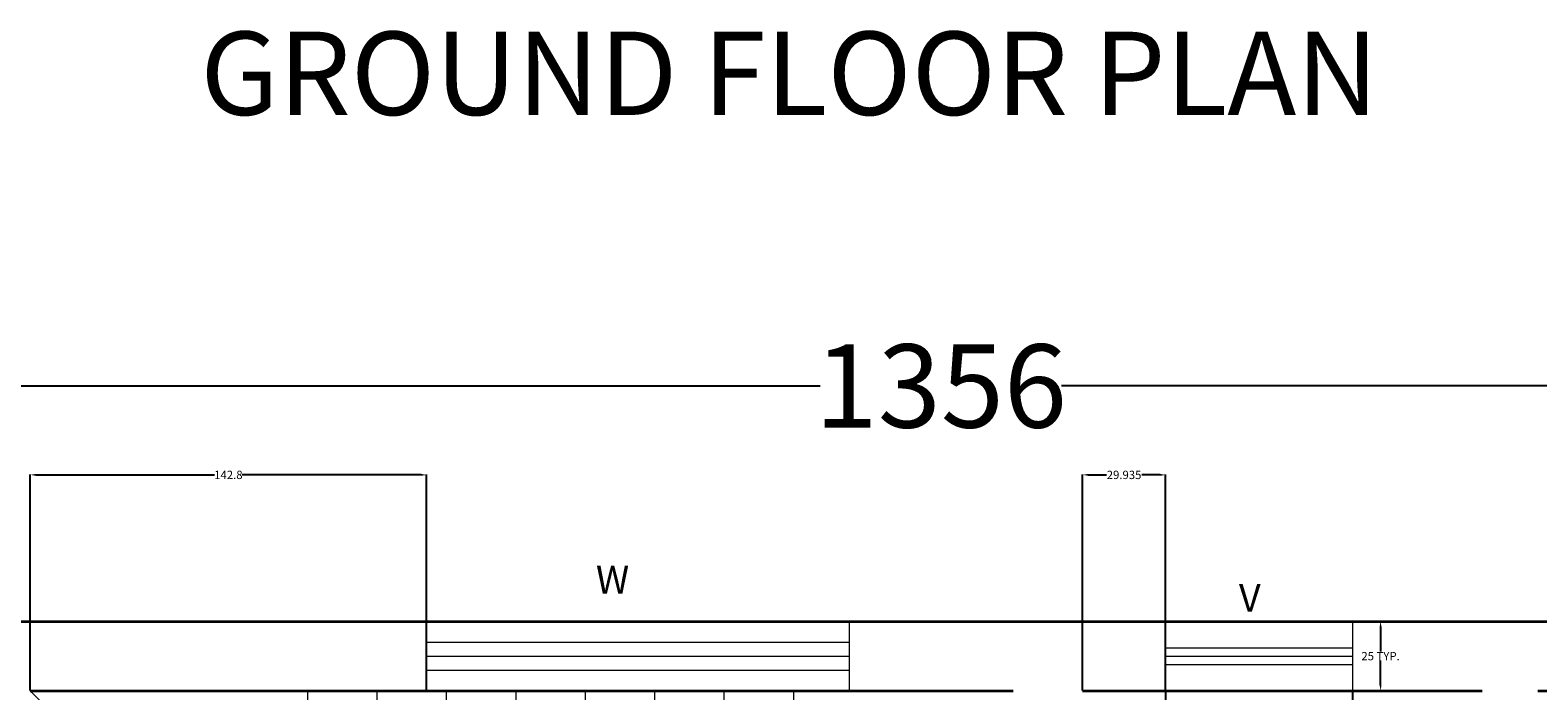
# Model space of a CAD drawing. Units: centimetres. Extents: x -121 to 3851, y -16 to 1180.
# Tile 6 of 16: x 415 to 958, y 855 to 1093. Entities that reach past the tile are written whole.
import ezdxf

# ---------------------------------------------------------------- set-up
doc = ezdxf.new("R2010")
doc.units = ezdxf.units.CM
doc.header["$MEASUREMENT"] = 0
for name, color, linetype, lineweight in [('A-ANNO-DIMS', 2, 'Continuous', 18), ('A-ANNO-IDEN', 3, 'Continuous', 13), ('A-ANNO-TEXT', 7, 'Continuous', 25), ('A-FLOR-STRS', 3, 'Continuous', 18), ('A-GLAZ', 4, 'Continuous', 18), ('A-WALL', 7, 'Continuous', 35)]:
    doc.layers.add(name, color=color, linetype=linetype, lineweight=lineweight)
doc.styles.get("Standard").update_dxf_attribs({"font": 'arial.ttf'})
doc.dimstyles.get("Standard").update_dxf_attribs({"dimtxt": 3, "dimasz": 2, "dimexe": 0.18, "dimexo": 0.0625, "dimgap": 0.09, "dimtad": 0, "dimtih": 1, "dimtoh": 1, "dimdec": 0, "dimzin": 0, "dimdsep": 46, "dimtxsty": 'Standard', "dimcen": 0.09, "dimadec": 0, "dimazin": 0, "dimtfac": 1, "dimtdec": 0, "dimtofl": 0, "dimtmove": 0, "dimatfit": 3, "dimfxl": 1, "dimtolj": 1, "dimtzin": 0, "dimarcsym": 0})

# ---------------------------------------------------------------- blocks, each defined once
blk = doc.blocks.new('*D1')
at = {"layer": 'A-ANNO-DIMS', "color": 0, "lineweight": -2, "transparency": 16777216}
for p, q in [((65.04, 880.08), (65.04, 964.95)), ((67.04, 964.77), (699.58, 964.77)), ((1419.04, 964.77), (786.5, 964.77)), ((1421.04, 880.08), (1421.04, 964.95))]:
    blk.add_line(p, q, dxfattribs=at)
at = {"layer": 'A-ANNO-DIMS', "color": 0, "transparency": 16777216}
for points in [[(67.04, 965.1), (67.04, 964.43), (65.04, 964.77)], [(1419.04, 965.1), (1419.04, 964.43), (1421.04, 964.77)]]:
    blk.add_solid(points, dxfattribs=at)
at = {"layer": 'Defpoints', "color": 0, "transparency": 16777216}
for p in [(1421.04, 964.77), (65.04, 880.01), (1421.04, 880.01)]:
    blk.add_point(p, dxfattribs=at)
at = {"layer": 'A-ANNO-DIMS', "color": 0, "transparency": 16777216, "insert": (743.04, 964.77), "char_height": 3, "attachment_point": 5}
blk.add_mtext('\\A1;{\\H10x;1356}', dxfattribs=at)
blk = doc.blocks.new('WIN-152CM')
for p, q in [((0, 17.5), (152.19, 17.5)), ((0, 12.5), (152.19, 12.5)), ((0, 7.5), (152.19, 7.5))]:
    blk.add_line(p, q)
blk.add_lwpolyline([(0, 25), (152.19, 25), (152.19, 0), (0, 0)], close=True)
blk = doc.blocks.new('VENT-67CM')
for p, q in [((0, 15.5), (67.32, 15.5)), ((0, 12.5), (67.32, 12.5)), ((0, 9.5), (67.32, 9.5))]:
    blk.add_line(p, q)
blk.add_lwpolyline([(0, 25), (67.32, 25), (67.32, 0), (0, 0)], close=True)
blk = doc.blocks.new('STAIR-L-RETURN')
for p, q in [((0, 225), (99.13, 125)), ((100, 100), (100, 225)), ((125, 125), (125, 225)), ((150, 125), (150, 225)), ((175, 125), (175, 225)), ((200, 125), (200, 225)), ((225, 125), (225, 225)), ((250, 125), (250, 225)), ((275, 125), (275, 225)), ((0, 125), (99.13, 125)), ((99.13, 125), (354, 125)), ((100, 0), (100, 125)), ((0, 100), (100, 100)), ((0, 75), (100, 75)), ((0, 50), (100, 50)), ((0, 25), (100, 25)), ((0, 0), (100, 0))]:
    blk.add_line(p, q)
blk = doc.blocks.new('*D29')
at = {"layer": 'A-ANNO-DIMS', "color": 0, "lineweight": -2, "transparency": 16777216}
for p, q in [((823.97, 854.95), (823.97, 844.74)), ((891.29, 854.95), (891.29, 844.74)), ((825.97, 844.92), (843.99, 844.92)), ((889.29, 844.92), (871.27, 844.92))]:
    blk.add_line(p, q, dxfattribs=at)
at = {"layer": 'A-ANNO-DIMS', "color": 0, "transparency": 16777216}
for points in [[(825.97, 845.25), (825.97, 844.58), (823.97, 844.92)], [(889.29, 845.25), (889.29, 844.58), (891.29, 844.92)]]:
    blk.add_solid(points, dxfattribs=at)
at = {"layer": 'Defpoints', "color": 0, "transparency": 16777216}
for p in [(823.97, 855.01), (891.29, 855.01), (891.29, 844.92)]:
    blk.add_point(p, dxfattribs=at)
at = {"layer": 'A-ANNO-DIMS', "color": 0, "transparency": 16777216, "insert": (857.63, 844.92), "char_height": 3, "attachment_point": 5}
blk.add_mtext('\\A1;VENT 67 TYP.', dxfattribs=at)
blk = doc.blocks.new('*D30')
at = {"layer": 'A-ANNO-DIMS', "color": 0, "lineweight": -2, "transparency": 16777216}
for p, q in [((891.36, 880.01), (901.57, 880.01)), ((901.39, 878.01), (901.39, 869.14)), ((901.39, 857.01), (901.39, 865.89)), ((891.36, 855.01), (901.57, 855.01))]:
    blk.add_line(p, q, dxfattribs=at)
at = {"layer": 'A-ANNO-DIMS', "color": 0, "transparency": 16777216}
for points in [[(901.06, 878.01), (901.73, 878.01), (901.39, 880.01)], [(901.06, 857.01), (901.73, 857.01), (901.39, 855.01)]]:
    blk.add_solid(points, dxfattribs=at)
at = {"layer": 'Defpoints', "color": 0, "transparency": 16777216}
for p in [(891.29, 880.01), (901.39, 880.01), (891.29, 855.01)]:
    blk.add_point(p, dxfattribs=at)
at = {"layer": 'A-ANNO-DIMS', "color": 0, "transparency": 16777216, "insert": (901.39, 867.51), "char_height": 3, "attachment_point": 5}
blk.add_mtext('\\A1;25 TYP.', dxfattribs=at)
blk = doc.blocks.new('*D53')
at = {"layer": 'A-ANNO-DIMS', "color": 0, "lineweight": -2, "transparency": 16777216}
for p, q in [((794.04, 855.08), (794.04, 932.94)), ((796.04, 932.76), (802.65, 932.76)), ((821.97, 932.76), (815.36, 932.76)), ((823.97, 855.08), (823.97, 932.94))]:
    blk.add_line(p, q, dxfattribs=at)
at = {"layer": 'A-ANNO-DIMS', "color": 0, "transparency": 16777216}
for points in [[(796.04, 933.1), (796.04, 932.43), (794.04, 932.76)], [(821.97, 933.1), (821.97, 932.43), (823.97, 932.76)]]:
    blk.add_solid(points, dxfattribs=at)
at = {"layer": 'Defpoints', "color": 0, "transparency": 16777216}
for p in [(823.97, 932.76), (794.04, 855.01), (823.97, 855.01)]:
    blk.add_point(p, dxfattribs=at)
at = {"layer": 'A-ANNO-DIMS', "color": 0, "transparency": 16777216, "insert": (809.01, 932.76), "char_height": 3, "attachment_point": 5}
blk.add_mtext('\\A1;29.935', dxfattribs=at)
blk = doc.blocks.new('*D63')
at = {"layer": 'A-ANNO-DIMS', "color": 0, "lineweight": -2, "transparency": 16777216}
for p, q in [((415.04, 855.08), (415.04, 932.94)), ((417.04, 932.76), (481.42, 932.76)), ((555.83, 932.76), (491.45, 932.76)), ((557.83, 855.08), (557.83, 932.94))]:
    blk.add_line(p, q, dxfattribs=at)
at = {"layer": 'A-ANNO-DIMS', "color": 0, "transparency": 16777216}
for points in [[(417.04, 933.1), (417.04, 932.43), (415.04, 932.76)], [(555.83, 933.1), (555.83, 932.43), (557.83, 932.76)]]:
    blk.add_solid(points, dxfattribs=at)
at = {"layer": 'Defpoints', "color": 0, "transparency": 16777216}
for p in [(557.83, 932.76), (415.04, 855.01), (557.83, 855.01)]:
    blk.add_point(p, dxfattribs=at)
at = {"layer": 'A-ANNO-DIMS', "color": 0, "transparency": 16777216, "insert": (486.43, 932.76), "char_height": 3, "attachment_point": 5}
blk.add_mtext('\\A1;142.8', dxfattribs=at)

msp = doc.modelspace()

# ---------------------------------------------------------------- linework, layer by layer
at = {"layer": 'A-WALL'}
for p, q in [((390.0382, 880.0141), (1421.0382, 880.0141)), ((415.0382, 855.0141), (769.0382, 855.0141)), ((794.0382, 855.0141), (938.0382, 855.0141)), ((958.0382, 855.0141), (1396.0382, 855.0141))]:
    msp.add_line(p, q, dxfattribs=at)

# ---------------------------------------------------------------- block references
at = {"layer": 'A-FLOR-STRS'}
msp.add_blockref('STAIR-L-RETURN', (415.038, 630.014), dxfattribs=at)
at = {"layer": 'A-GLAZ'}
for name, p in [('WIN-152CM', (557.8305, 855.014)), ('VENT-67CM', (823.973, 855.014))]:
    msp.add_blockref(name, p, dxfattribs=at)

# ---------------------------------------------------------------- texts
at = {"layer": 'A-ANNO-IDEN', "char_height": 10, "attachment_point": 1}
for s, insert in [('W', (618.8013, 900.0527)), ('V', (850.3746, 893.5113))]:
    msp.add_mtext_dynamic_manual_height_columns(s, width=55.718495, gutter_width=1, heights=[0], dxfattribs=dict(at, insert=insert))
at = {"layer": 'A-ANNO-TEXT', "insert": (476.3488, 1092.339), "char_height": 30, "attachment_point": 1}
msp.add_mtext_dynamic_manual_height_columns('GROUND FLOOR PLAN', width=1207.704783, gutter_width=1, heights=[0], dxfattribs=at)

# ---------------------------------------------------------------- dimensions: what is measured, and where the dimension line sits
at = {"layer": 'A-ANNO-DIMS'}
for base, p1, p2, text, override, picture, middle in [((1421.0382, 964.7682), (65.0382, 880.0141), (1421.0382, 880.0141), '{\\H10x;<>}', {"dimclrd": 0, "dimclre": 0, "dimclrt": 0}, '*D1', (743.0382, 964.7682)), ((891.2948, 844.9158), (823.973, 855.0141), (891.2948, 855.0141), 'VENT <> TYP.', {"dimdec": 0, "dimlfac": 1, "dimrnd": 0, "dimzin": 0, "dimdsep": 46, "dimlunit": 2}, '*D29', (857.6339, 844.9158))]:
    dim = msp.add_linear_dim(base=base, p1=p1, p2=p2, text=text, dimstyle='Standard', override=override, dxfattribs=at)
    dim.commit()
    dim.dimension.update_dxf_attribs({"geometry": picture, "text_midpoint": middle})
dim = msp.add_linear_dim(base=(557.8306, 932.7641), p1=(415.0382, 855.0141), p2=(557.8306, 855.0141), angle=0, dimstyle='Standard', override={"dimdec": 1, "dimlfac": 1, "dimrnd": 0, "dimzin": 0, "dimdsep": 46, "dimlunit": 2}, dxfattribs=at)
dim.commit()
dim.dimension.update_dxf_attribs({"geometry": '*D63', "text_midpoint": (486.4344, 932.7641)})
dim = msp.add_linear_dim(base=(823.973, 932.7641), p1=(794.0382, 855.0141), p2=(823.973, 855.0141), dimstyle='Standard', override={"dimdec": 3, "dimlfac": 1, "dimrnd": 0, "dimzin": 0, "dimdsep": 46, "dimlunit": 2}, dxfattribs=at)
dim.commit()
dim.dimension.update_dxf_attribs({"geometry": '*D53', "text_midpoint": (809.0056, 932.7641)})
dim = msp.add_linear_dim(base=(901.3931, 880.0141), p1=(891.2948, 855.0141), p2=(891.2948, 880.0141), angle=90, text='<> TYP.', dimstyle='Standard', override={"dimdec": 0, "dimlfac": 1, "dimrnd": 0, "dimzin": 0, "dimdsep": 46, "dimlunit": 2}, dxfattribs=at)
dim.commit()
dim.dimension.update_dxf_attribs({"geometry": '*D30', "text_midpoint": (901.3931, 867.5141)})

doc.saveas('drawing.dxf')
